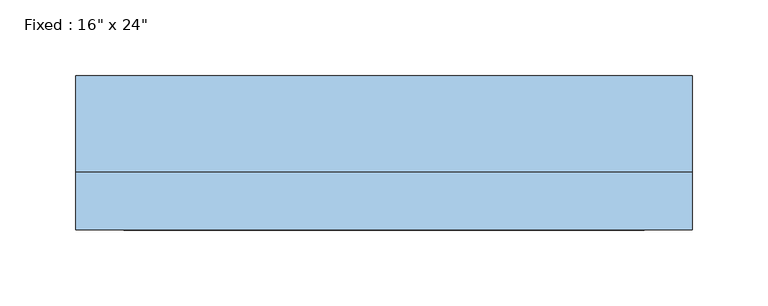
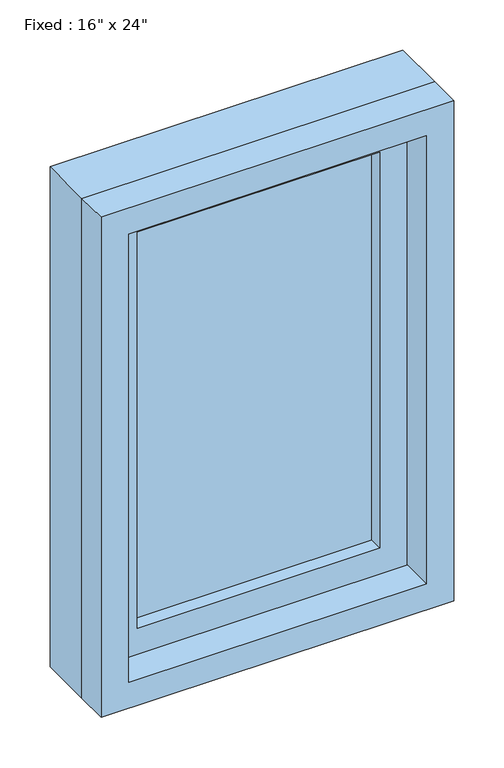
"""IFC4 building model written with IfcOpenShell, lengths in millimetres: window geometry."""

from ifc_helpers import new_model, si_unit, frame, origin, place, context, project, spatial, polyline, outline, extrude, source, transform, mapped, element, save


def window_a112695e(model_context):
    return source(origin(), model_context, "Body", "SweptSolid", [
        extrude(outline(polyline([(101.6, 3.175), (-177.8, 3.175), (-177.8, 15.875), (101.6, 15.875), (101.6, 3.175)])), frame((0.0, 0.0, 977.9), z_axis=(0.0, 0.0, 1.0), x_axis=(1.0, 0.0, 0.0)), (0.0, 0.0, 1.0), 482.6),
        extrude(outline(polyline([(1504.95, -222.25), (933.45, -222.25), (933.45, 146.05), (1504.95, 146.05), (1504.95, -222.25)]), holes=[polyline([(1460.5, -177.8), (1460.5, 101.6), (977.9, 101.6), (977.9, -177.8), (1460.5, -177.8)])]), frame((0.0, -12.7, 0.0), z_axis=(0.0, 1.0, 0.0), x_axis=(0.0, 0.0, 1.0)), (0.0, 0.0, 1.0), 44.45),
        extrude(outline(polyline([(1524.0, -241.3), (914.4, -241.3), (914.4, 165.1), (1524.0, 165.1), (1524.0, -241.3)]), holes=[polyline([(1492.25, -209.55), (1492.25, 133.35), (946.15, 133.35), (946.15, -209.55), (1492.25, -209.55)])]), frame((0.0, -50.8, 0.0), z_axis=(0.0, 1.0, 0.0), x_axis=(0.0, 0.0, 1.0)), (0.0, 0.0, 1.0), 38.1),
        extrude(outline(polyline([(1524.0, 165.1), (1524.0, -241.3), (914.4, -241.3), (914.4, 165.1), (1524.0, 165.1)]), holes=[polyline([(1504.95, 146.05), (933.45, 146.05), (933.45, -222.25), (1504.95, -222.25), (1504.95, 146.05)])]), frame((0.0, -12.7, 0.0), z_axis=(0.0, 1.0, 0.0), x_axis=(0.0, 0.0, 1.0)), (0.0, 0.0, 1.0), 63.5),
    ])


if __name__ == "__main__":
    model = new_model("IFC4")
    model_context = context("Model", 3, world=origin())
    ifc_project = project(units=[si_unit("LENGTHUNIT", "METRE", prefix="MILLI")], contexts=[model_context])
    site = spatial("IfcSite", under=ifc_project)
    building = spatial("IfcBuilding", under=site)
    placement = place(None, origin())
    window_shape = window_a112695e(model_context)
    element("IfcWindow", 1, ObjectType="Fixed : 16\" x 24\"", at=placement, inside=building, context=model_context, shape_type="MappedRepresentation", body=[
        mapped(window_shape, transform((0.0, 0.0, 0.0), x_axis=(1.0, 0.0, 0.0), y_axis=(0.0, 1.0, 0.0), z_axis=(0.0, 0.0, 1.0))),
    ])
    save(model, "model.ifc")

# Revit data of these elements
# Type "Fixed : 16\" x 24\""
#   Type Mark = "4"
#   Construction Type Id = "GSP4R"
#   Assembly Code = "B2020100"
#   Analytic Construction = "1/8 in Pilkington single glazing"
#   Visual Light Transmittance = 0.9
#   Solar Heat Gain Coefficient = 0.78
#   Heat Transfer Coefficient (U) = 0.6496 BTU/(h·ft²·°F)
#   Height = 2' - 0"
#   Default Sill Height = 3' - 0"
#   Width = 1' - 4"
#   Window Inset = 0' - 0 3/4"
#   Define Thermal Properties by = 1
#   Glass Pane Material = Glass
#   Sash Material = Sash
#   Wall Closure = (empty or 0)
# Element 1 (IfcWindow, "Fixed : 16\" x 24\"")
#   Materials on its faces: "Sash", "Glass"
# Materials
#   "Glass": class "Glass", colour RGB 0 128 192, transparency 0.75, Description = "Soda Lime Glass", Cost = 0
#   "Sash": class "Wood", colour RGB 224 178 126, transparency 0
